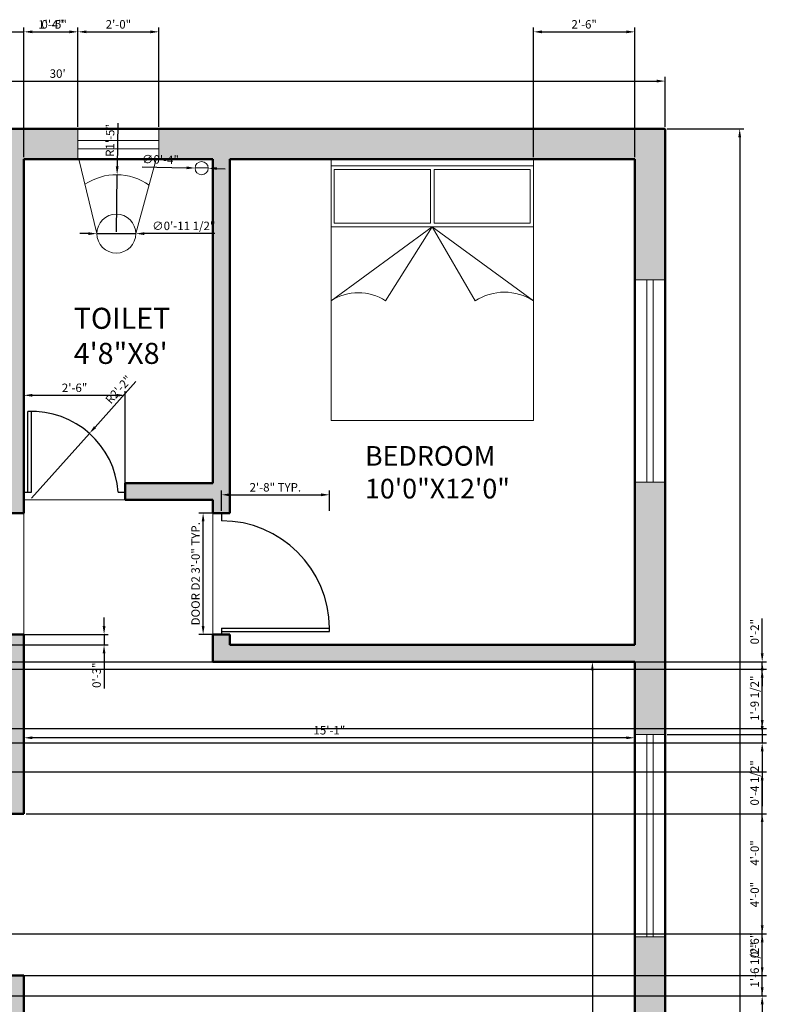
# Model space of a CAD drawing. Units: inches. Extents: x 457 to 882, y 0 to 1111.
# Tile 4 of 4: x 660 to 882, y 817 to 1109. Entities that reach past the tile are written whole.
import ezdxf

# ---------------------------------------------------------------- set-up
doc = ezdxf.new("R2010")
doc.units = ezdxf.units.IN
for name, color, linetype, lineweight in [('A-ANNO-DIMS', 2, 'Continuous', 18), ('A-AREA-IDEN', 7, 'Continuous', 25), ('A-DOOR', 3, 'Continuous', 25), ('A-DOOR-THRE', 8, 'Continuous', 13), ('A-FLOR-FIXT', 8, 'Continuous', 18), ('A-FURN', 8, 'Continuous', 18), ('A-GLAZ', 5, 'Continuous', 18), ('A-WALL', 7, 'Continuous', 50), ('A-WALL-PATT', 252, 'Continuous', 13)]:
    doc.layers.add(name, color=color, linetype=linetype, lineweight=lineweight)
doc.styles.get("Standard").update_dxf_attribs({"font": 'arial.ttf'})
doc.dimstyles.new('ISO-25', dxfattribs={"dimtxt": 2.5, "dimasz": 2.5, "dimexe": 1.25, "dimexo": 0.625, "dimtad": 1, "dimdec": 0, "dimlunit": 3, "dimtxsty": 'Standard', "dimcen": 2.5, "dimadec": 0, "dimazin": 0, "dimtfac": 1, "dimtdec": 0, "dimtmove": 0, "dimatfit": 3, "dimfxl": 1, "dimarcsym": 0})

# ---------------------------------------------------------------- blocks, each defined once
blk = doc.blocks.new('*D2')
at = {"layer": 'A-ANNO-DIMS', "color": 0, "lineweight": -2, "transparency": 16777216}
for p, q in [((491.26, 1077.13), (491.26, 1091.91)), ((851.26, 1077.13), (851.26, 1091.91)), ((493.76, 1090.66), (848.76, 1090.66))]:
    blk.add_line(p, q, dxfattribs=at)
at = {"layer": 'A-ANNO-DIMS', "color": 0, "transparency": 16777216}
for points in [[(493.76, 1091.08), (493.76, 1090.24), (491.26, 1090.66)], [(848.76, 1091.08), (848.76, 1090.24), (851.26, 1090.66)]]:
    blk.add_solid(points, dxfattribs=at)
at = {"layer": 'Defpoints', "color": 0, "transparency": 16777216}
for p in [(851.26, 1090.66), (491.26, 1076.51), (851.26, 1076.51)]:
    blk.add_point(p, dxfattribs=at)
at = {"layer": 'A-ANNO-DIMS', "color": 0, "transparency": 16777216, "insert": (671.26, 1092.56), "char_height": 2.5, "attachment_point": 5}
blk.add_mtext("30'", dxfattribs=at)
blk = doc.blocks.new('*D3')
at = {"layer": 'A-ANNO-DIMS', "color": 0, "lineweight": -2, "transparency": 16777216}
for p, q in [((851.88, 1076.51), (874.6, 1076.51)), ((873.35, 1074.01), (873.35, 539.01)), ((851.88, 536.51), (874.6, 536.51))]:
    blk.add_line(p, q, dxfattribs=at)
at = {"layer": 'A-ANNO-DIMS', "color": 0, "transparency": 16777216}
for points in [[(872.93, 1074.01), (873.76, 1074.01), (873.35, 1076.51)], [(872.93, 539.01), (873.76, 539.01), (873.35, 536.51)]]:
    blk.add_solid(points, dxfattribs=at)
at = {"layer": 'Defpoints', "color": 0, "transparency": 16777216}
for p in [(851.26, 1076.51), (851.26, 536.51), (873.35, 536.51)]:
    blk.add_point(p, dxfattribs=at)
at = {"layer": 'A-ANNO-DIMS', "color": 0, "transparency": 16777216, "insert": (871.45, 806.51), "char_height": 2.5, "attachment_point": 5, "rotation": 90}
blk.add_mtext("45'", dxfattribs=at)
blk = doc.blocks.new('*D6')
at = {"layer": 'A-ANNO-DIMS', "color": 0, "lineweight": -2, "transparency": 16777216}
for p, q in [((661.26, 917.88), (661.26, 894.76)), ((842.26, 917.88), (842.26, 894.76)), ((839.76, 896.01), (663.76, 896.01))]:
    blk.add_line(p, q, dxfattribs=at)
at = {"layer": 'A-ANNO-DIMS', "color": 0, "transparency": 16777216}
for points in [[(663.76, 896.42), (663.76, 895.59), (661.26, 896.01)], [(839.76, 896.42), (839.76, 895.59), (842.26, 896.01)]]:
    blk.add_solid(points, dxfattribs=at)
at = {"layer": 'Defpoints', "color": 0, "transparency": 16777216}
for p in [(661.26, 918.51), (842.26, 918.51), (661.26, 896.01)]:
    blk.add_point(p, dxfattribs=at)
at = {"layer": 'A-ANNO-DIMS', "color": 0, "transparency": 16777216, "insert": (751.76, 897.91), "char_height": 2.5, "attachment_point": 5}
blk.add_mtext('15\'-1"', dxfattribs=at)
blk = doc.blocks.new('*D7')
at = {"layer": 'A-ANNO-DIMS', "color": 0, "lineweight": -2, "transparency": 16777216}
for p, q in [((841.63, 918.51), (828.45, 918.51)), ((829.7, 916.01), (829.7, 631.01)), ((841.63, 628.51), (828.45, 628.51))]:
    blk.add_line(p, q, dxfattribs=at)
at = {"layer": 'A-ANNO-DIMS', "color": 0, "transparency": 16777216}
for points in [[(829.28, 916.01), (830.11, 916.01), (829.7, 918.51)], [(829.28, 631.01), (830.11, 631.01), (829.7, 628.51)]]:
    blk.add_solid(points, dxfattribs=at)
at = {"layer": 'Defpoints', "color": 0, "transparency": 16777216}
for p in [(842.26, 918.51), (829.7, 628.51), (842.26, 628.51)]:
    blk.add_point(p, dxfattribs=at)
at = {"layer": 'A-ANNO-DIMS', "color": 0, "transparency": 16777216, "insert": (827.82, 773.51), "char_height": 2.5, "attachment_point": 5, "rotation": 90}
blk.add_mtext('24\'-2"', dxfattribs=at)
blk = doc.blocks.new('BED-DOUBLE-60')
for p, q in [((0, 77.49), (0, 0)), ((60, 77.49), (0, 77.49)), ((60, 0), (60, 77.49)), ((60, 75.49), (0, 75.49)), ((29.44, 74.49), (0.94, 74.49)), ((0.94, 74.49), (0.94, 58.49)), ((29.44, 74.49), (29.44, 58.49)), ((59, 74.49), (30.53, 74.49)), ((30.53, 74.49), (30.53, 58.49)), ((59, 74.49), (59, 58.49)), ((29.44, 58.49), (0.94, 58.49)), ((59, 58.49), (30.53, 58.49)), ((60, 57.49), (0, 57.49)), ((30, 57.49), (0, 35.49)), ((30, 57.49), (16.16, 35.49)), ((60, 35.49), (30, 57.49)), ((30, 57.49), (42.73, 35.49)), ((0, 0), (60, 0))]:
    blk.add_line(p, q)
for centre, radius, start, end in [((51.36, 22.4), 15.69, 56.5972, 123.4028), ((8.08, 23.34), 14.59, 56.3669, 123.6331)]:
    blk.add_arc(centre, radius, start, end)
blk = doc.blocks.new('WIN-60-GLAZING')
for p, q in [((0, 0), (0, 60)), ((1.86, 0), (1.86, 60))]:
    blk.add_line(p, q)
blk = doc.blocks.new('DOOR-32-SWING')
for p, q in [((0, 36), (0, 33.7)), ((0, 1.85), (32, 1.85)), ((0, 1.85), (0, 0))]:
    blk.add_line(p, q)
blk.add_arc((0, 1.7), 32, 0.2643, 90)
blk = doc.blocks.new('*D20')
at = {"layer": 'A-ANNO-DIMS', "color": 0, "lineweight": -2, "transparency": 16777216}
for p, q in [((719.13, 962.63), (713.11, 962.63)), ((714.36, 929.13), (714.36, 960.13)), ((719.13, 926.63), (713.11, 926.63))]:
    blk.add_line(p, q, dxfattribs=at)
at = {"layer": 'A-ANNO-DIMS', "color": 0, "transparency": 16777216}
for points in [[(713.94, 960.13), (714.77, 960.13), (714.36, 962.63)], [(713.94, 929.13), (714.77, 929.13), (714.36, 926.63)]]:
    blk.add_solid(points, dxfattribs=at)
at = {"layer": 'Defpoints', "color": 0, "transparency": 16777216}
for p in [(714.36, 962.63), (719.76, 962.63), (719.76, 926.63)]:
    blk.add_point(p, dxfattribs=at)
at = {"layer": 'A-ANNO-DIMS', "color": 0, "transparency": 16777216, "insert": (712.44, 944.63), "char_height": 2.5, "attachment_point": 5, "rotation": 90}
blk.add_mtext('DOOR D2 3\'-0" TYP.', dxfattribs=at)
blk = doc.blocks.new('*D21')
at = {"layer": 'A-ANNO-DIMS', "color": 0, "lineweight": -2, "transparency": 16777216}
for p, q in [((719.76, 963.25), (719.76, 969.28)), ((751.76, 963.25), (751.76, 969.28)), ((722.26, 968.03), (749.26, 968.03))]:
    blk.add_line(p, q, dxfattribs=at)
at = {"layer": 'A-ANNO-DIMS', "color": 0, "transparency": 16777216}
for points in [[(722.26, 968.45), (722.26, 967.61), (719.76, 968.03)], [(749.26, 968.45), (749.26, 967.61), (751.76, 968.03)]]:
    blk.add_solid(points, dxfattribs=at)
at = {"layer": 'Defpoints', "color": 0, "transparency": 16777216}
for p in [(751.76, 968.03), (719.76, 962.63), (751.76, 962.63)]:
    blk.add_point(p, dxfattribs=at)
at = {"layer": 'A-ANNO-DIMS', "color": 0, "transparency": 16777216, "insert": (735.76, 969.93), "char_height": 2.5, "attachment_point": 5}
blk.add_mtext('2\'-8" TYP.', dxfattribs=at)
blk = doc.blocks.new('*D24')
at = {"layer": 'A-ANNO-DIMS', "color": 0, "lineweight": -2, "transparency": 16777216}
for p, q in [((661.26, 969.4), (661.26, 998.77)), ((691.26, 969.4), (691.26, 998.77)), ((663.76, 997.52), (688.76, 997.52))]:
    blk.add_line(p, q, dxfattribs=at)
at = {"layer": 'A-ANNO-DIMS', "color": 0, "transparency": 16777216}
for points in [[(663.76, 997.94), (663.76, 997.1), (661.26, 997.52)], [(688.76, 997.94), (688.76, 997.1), (691.26, 997.52)]]:
    blk.add_solid(points, dxfattribs=at)
at = {"layer": 'Defpoints', "color": 0, "transparency": 16777216}
for p in [(691.26, 997.52), (661.26, 968.77), (691.26, 968.77)]:
    blk.add_point(p, dxfattribs=at)
at = {"layer": 'A-ANNO-DIMS', "color": 0, "transparency": 16777216, "insert": (676.26, 999.42), "char_height": 2.5, "attachment_point": 5}
blk.add_mtext('2\'-6"', dxfattribs=at)
blk = doc.blocks.new('*D27')
at = {"layer": 'A-ANNO-DIMS', "color": 0, "lineweight": -2, "transparency": 16777216}
for p, q in [((685.01, 929.13), (685.01, 931.63)), ((656.88, 926.63), (686.26, 926.63)), ((685.01, 926.63), (685.01, 923.51)), ((656.88, 923.51), (686.26, 923.51)), ((685.01, 921.01), (685.01, 910.61))]:
    blk.add_line(p, q, dxfattribs=at)
at = {"layer": 'A-ANNO-DIMS', "color": 0, "transparency": 16777216}
for points in [[(684.59, 929.13), (685.42, 929.13), (685.01, 926.63)], [(684.59, 921.01), (685.42, 921.01), (685.01, 923.51)]]:
    blk.add_solid(points, dxfattribs=at)
at = {"layer": 'Defpoints', "color": 0, "transparency": 16777216}
for p in [(656.26, 926.63), (656.26, 923.51), (685.01, 923.51)]:
    blk.add_point(p, dxfattribs=at)
at = {"layer": 'A-ANNO-DIMS', "color": 0, "transparency": 16777216, "insert": (683.11, 914.56), "char_height": 2.5, "attachment_point": 5, "rotation": 90}
blk.add_mtext('0\'-3"', dxfattribs=at)
blk = doc.blocks.new('*D29')
at = {"layer": 'A-ANNO-DIMS', "color": 0, "lineweight": -2, "transparency": 16777216}
for p, q in [((656.26, 1068.13), (656.26, 1106.51)), ((661.26, 1068.13), (661.26, 1106.51)), ((653.76, 1105.26), (651.26, 1105.26)), ((656.26, 1105.26), (661.26, 1105.26)), ((663.76, 1105.26), (674.15, 1105.26))]:
    blk.add_line(p, q, dxfattribs=at)
at = {"layer": 'A-ANNO-DIMS', "color": 0, "transparency": 16777216}
for points in [[(653.76, 1105.67), (653.76, 1104.84), (656.26, 1105.26)], [(663.76, 1105.67), (663.76, 1104.84), (661.26, 1105.26)]]:
    blk.add_solid(points, dxfattribs=at)
at = {"layer": 'Defpoints', "color": 0, "transparency": 16777216}
for p in [(661.26, 1105.26), (656.26, 1067.51), (661.26, 1067.51)]:
    blk.add_point(p, dxfattribs=at)
at = {"layer": 'A-ANNO-DIMS', "color": 0, "transparency": 16777216, "insert": (670.21, 1107.16), "char_height": 2.5, "attachment_point": 5}
blk.add_mtext('0\'-5"', dxfattribs=at)
blk = doc.blocks.new('*D34')
at = {"layer": 'A-ANNO-DIMS', "color": 0, "lineweight": -2, "transparency": 16777216}
for p, q in [((842.88, 918.51), (881.26, 918.51)), ((880.01, 899.48), (880.01, 916.01)), ((851.88, 896.98), (881.26, 896.98))]:
    blk.add_line(p, q, dxfattribs=at)
at = {"layer": 'A-ANNO-DIMS', "color": 0, "transparency": 16777216}
for points in [[(879.59, 916.01), (880.42, 916.01), (880.01, 918.51)], [(879.59, 899.48), (880.42, 899.48), (880.01, 896.98)]]:
    blk.add_solid(points, dxfattribs=at)
at = {"layer": 'Defpoints', "color": 0, "transparency": 16777216}
for p in [(842.26, 918.51), (880.01, 918.51), (851.26, 896.98)]:
    blk.add_point(p, dxfattribs=at)
at = {"layer": 'A-ANNO-DIMS', "color": 0, "transparency": 16777216, "insert": (878.09, 907.74), "char_height": 2.5, "attachment_point": 5, "rotation": 90}
blk.add_mtext('1\'-9 1/2"', dxfattribs=at)
blk = doc.blocks.new('*D36')
at = {"layer": 'A-ANNO-DIMS', "color": 0, "lineweight": -2, "transparency": 16777216}
for p, q in [((661.26, 1068.13), (661.26, 1106.51)), ((677.26, 1077.13), (677.26, 1106.51)), ((663.76, 1105.26), (674.76, 1105.26))]:
    blk.add_line(p, q, dxfattribs=at)
at = {"layer": 'A-ANNO-DIMS', "color": 0, "transparency": 16777216}
for points in [[(663.76, 1105.67), (663.76, 1104.84), (661.26, 1105.26)], [(674.76, 1105.67), (674.76, 1104.84), (677.26, 1105.26)]]:
    blk.add_solid(points, dxfattribs=at)
at = {"layer": 'Defpoints', "color": 0, "transparency": 16777216}
for p in [(677.26, 1105.26), (677.26, 1076.51), (661.26, 1067.51)]:
    blk.add_point(p, dxfattribs=at)
at = {"layer": 'A-ANNO-DIMS', "color": 0, "transparency": 16777216, "insert": (669.26, 1107.14), "char_height": 2.5, "attachment_point": 5}
blk.add_mtext('1\'-4"', dxfattribs=at)
blk = doc.blocks.new('*D37')
at = {"layer": 'A-ANNO-DIMS', "color": 0, "lineweight": -2, "transparency": 16777216}
for p, q in [((677.26, 1077.13), (677.26, 1106.51)), ((701.26, 1077.13), (701.26, 1106.51)), ((679.76, 1105.26), (698.76, 1105.26))]:
    blk.add_line(p, q, dxfattribs=at)
at = {"layer": 'A-ANNO-DIMS', "color": 0, "transparency": 16777216}
for points in [[(679.76, 1105.67), (679.76, 1104.84), (677.26, 1105.26)], [(698.76, 1105.67), (698.76, 1104.84), (701.26, 1105.26)]]:
    blk.add_solid(points, dxfattribs=at)
at = {"layer": 'Defpoints', "color": 0, "transparency": 16777216}
for p in [(701.26, 1105.26), (677.26, 1076.51), (701.26, 1076.51)]:
    blk.add_point(p, dxfattribs=at)
at = {"layer": 'A-ANNO-DIMS', "color": 0, "transparency": 16777216, "insert": (689.26, 1107.16), "char_height": 2.5, "attachment_point": 5}
blk.add_mtext('2\'-0"', dxfattribs=at)
blk = doc.blocks.new('*D47')
at = {"layer": 'A-ANNO-DIMS', "color": 0, "lineweight": -2, "transparency": 16777216}
for p, q in [((661.88, 873.51), (881.26, 873.51)), ((880.01, 828.01), (880.01, 871.01)), ((661.88, 825.51), (881.26, 825.51))]:
    blk.add_line(p, q, dxfattribs=at)
at = {"layer": 'A-ANNO-DIMS', "color": 0, "transparency": 16777216}
for points in [[(879.59, 871.01), (880.42, 871.01), (880.01, 873.51)], [(879.59, 828.01), (880.42, 828.01), (880.01, 825.51)]]:
    blk.add_solid(points, dxfattribs=at)
at = {"layer": 'Defpoints', "color": 0, "transparency": 16777216}
for p in [(661.26, 873.51), (880.01, 873.51), (661.26, 825.51)]:
    blk.add_point(p, dxfattribs=at)
at = {"layer": 'A-ANNO-DIMS', "color": 0, "transparency": 16777216, "insert": (878.11, 849.51), "char_height": 2.5, "attachment_point": 5, "rotation": 90}
blk.add_mtext('4\'-0"', dxfattribs=at)
blk = doc.blocks.new('*D48')
at = {"layer": 'A-ANNO-DIMS', "color": 0, "lineweight": -2, "transparency": 16777216}
for p, q in [((880.01, 828.01), (880.01, 838.4)), ((656.88, 825.51), (881.26, 825.51)), ((880.01, 819.51), (880.01, 825.51)), ((656.88, 819.51), (881.26, 819.51)), ((880.01, 817.01), (880.01, 814.51))]:
    blk.add_line(p, q, dxfattribs=at)
at = {"layer": 'A-ANNO-DIMS', "color": 0, "transparency": 16777216}
for points in [[(879.59, 828.01), (880.42, 828.01), (880.01, 825.51)], [(879.59, 817.01), (880.42, 817.01), (880.01, 819.51)]]:
    blk.add_solid(points, dxfattribs=at)
at = {"layer": 'Defpoints', "color": 0, "transparency": 16777216}
for p in [(656.26, 825.51), (880.01, 825.51), (656.26, 819.51)]:
    blk.add_point(p, dxfattribs=at)
at = {"layer": 'A-ANNO-DIMS', "color": 0, "transparency": 16777216, "insert": (878.11, 834.45), "char_height": 2.5, "attachment_point": 5, "rotation": 90}
blk.add_mtext('0\'-6"', dxfattribs=at)
blk = doc.blocks.new('*D50')
at = {"layer": 'A-ANNO-DIMS', "color": 0, "lineweight": -2, "transparency": 16777216}
for p, q in [((527.99, 885.87), (881.26, 885.87)), ((880.01, 840.37), (880.01, 883.37)), ((527.99, 837.87), (881.26, 837.87))]:
    blk.add_line(p, q, dxfattribs=at)
at = {"layer": 'A-ANNO-DIMS', "color": 0, "transparency": 16777216}
for points in [[(879.59, 883.37), (880.42, 883.37), (880.01, 885.87)], [(879.59, 840.37), (880.42, 840.37), (880.01, 837.87)]]:
    blk.add_solid(points, dxfattribs=at)
at = {"layer": 'Defpoints', "color": 0, "transparency": 16777216}
for p in [(527.36, 885.87), (880.01, 885.87), (527.36, 837.87)]:
    blk.add_point(p, dxfattribs=at)
at = {"layer": 'A-ANNO-DIMS', "color": 0, "transparency": 16777216, "insert": (878.11, 861.87), "char_height": 2.5, "attachment_point": 5, "rotation": 90}
blk.add_mtext('4\'-0"', dxfattribs=at)
blk = doc.blocks.new('*D51')
at = {"layer": 'A-ANNO-DIMS', "color": 0, "lineweight": -2, "transparency": 16777216}
for p, q in [((503.99, 837.87), (881.26, 837.87)), ((880.01, 822.01), (880.01, 835.37)), ((500.88, 819.51), (881.26, 819.51))]:
    blk.add_line(p, q, dxfattribs=at)
at = {"layer": 'A-ANNO-DIMS', "color": 0, "transparency": 16777216}
for points in [[(879.59, 835.37), (880.42, 835.37), (880.01, 837.87)], [(879.59, 822.01), (880.42, 822.01), (880.01, 819.51)]]:
    blk.add_solid(points, dxfattribs=at)
at = {"layer": 'Defpoints', "color": 0, "transparency": 16777216}
for p in [(503.36, 837.87), (880.01, 837.87), (500.26, 819.51)]:
    blk.add_point(p, dxfattribs=at)
at = {"layer": 'A-ANNO-DIMS', "color": 0, "transparency": 16777216, "insert": (878.09, 828.69), "char_height": 2.5, "attachment_point": 5, "rotation": 90}
blk.add_mtext('1\'-6 1/2"', dxfattribs=at)
blk = doc.blocks.new('*D55')
at = {"layer": 'A-ANNO-DIMS', "color": 0, "lineweight": -2, "transparency": 16777216}
for p, q in [((880.01, 921.01), (880.01, 931.4)), ((656.88, 918.51), (881.26, 918.51)), ((880.01, 916.3), (880.01, 918.51)), ((598.94, 916.3), (881.26, 916.3)), ((880.01, 913.8), (880.01, 911.3))]:
    blk.add_line(p, q, dxfattribs=at)
at = {"layer": 'A-ANNO-DIMS', "color": 0, "transparency": 16777216}
for points in [[(879.59, 921.01), (880.42, 921.01), (880.01, 918.51)], [(879.59, 913.8), (880.42, 913.8), (880.01, 916.3)]]:
    blk.add_solid(points, dxfattribs=at)
at = {"layer": 'Defpoints', "color": 0, "transparency": 16777216}
for p in [(656.26, 918.51), (880.01, 918.51), (598.31, 916.3)]:
    blk.add_point(p, dxfattribs=at)
at = {"layer": 'A-ANNO-DIMS', "color": 0, "transparency": 16777216, "insert": (878.11, 927.45), "char_height": 2.5, "attachment_point": 5, "rotation": 90}
blk.add_mtext('0\'-2"', dxfattribs=at)
blk = doc.blocks.new('*D57')
at = {"layer": 'A-ANNO-DIMS', "color": 0, "lineweight": -2, "transparency": 16777216}
for p, q in [((880.01, 901.27), (880.01, 903.77)), ((610.53, 898.77), (881.26, 898.77)), ((880.01, 898.77), (880.01, 894.51)), ((656.88, 894.51), (881.26, 894.51)), ((880.01, 892.01), (880.01, 875.78))]:
    blk.add_line(p, q, dxfattribs=at)
at = {"layer": 'A-ANNO-DIMS', "color": 0, "transparency": 16777216}
for points in [[(879.59, 901.27), (880.42, 901.27), (880.01, 898.77)], [(879.59, 892.01), (880.42, 892.01), (880.01, 894.51)]]:
    blk.add_solid(points, dxfattribs=at)
at = {"layer": 'Defpoints', "color": 0, "transparency": 16777216}
for p in [(609.9, 898.77), (656.26, 894.51), (880.01, 894.51)]:
    blk.add_point(p, dxfattribs=at)
at = {"layer": 'A-ANNO-DIMS', "color": 0, "transparency": 16777216, "insert": (878.09, 882.64), "char_height": 2.5, "attachment_point": 5, "rotation": 90}
blk.add_mtext('0\'-4 1/2"', dxfattribs=at)
blk = doc.blocks.new('*D59')
at = {"layer": 'A-ANNO-DIMS', "color": 0, "lineweight": -2, "transparency": 16777216}
for p, q in [((812.26, 1068.13), (812.26, 1106.51)), ((842.26, 1068.13), (842.26, 1106.51)), ((814.76, 1105.26), (839.76, 1105.26))]:
    blk.add_line(p, q, dxfattribs=at)
at = {"layer": 'A-ANNO-DIMS', "color": 0, "transparency": 16777216}
for points in [[(814.76, 1105.67), (814.76, 1104.84), (812.26, 1105.26)], [(839.76, 1105.67), (839.76, 1104.84), (842.26, 1105.26)]]:
    blk.add_solid(points, dxfattribs=at)
at = {"layer": 'Defpoints', "color": 0, "transparency": 16777216}
for p in [(842.26, 1105.26), (812.26, 1067.51), (842.26, 1067.51)]:
    blk.add_point(p, dxfattribs=at)
at = {"layer": 'A-ANNO-DIMS', "color": 0, "transparency": 16777216, "insert": (827.26, 1107.16), "char_height": 2.5, "attachment_point": 5}
blk.add_mtext('2\'-6"', dxfattribs=at)
blk = doc.blocks.new('*D62')
at = {"layer": 'A-ANNO-DIMS', "color": 0, "lineweight": -2, "transparency": 16777216}
for p, q in [((694.39, 1001.58), (682.33, 988.08)), ((663.49, 967), (680.66, 986.22))]:
    blk.add_line(p, q, dxfattribs=at)
at = {"layer": 'A-ANNO-DIMS', "color": 0, "transparency": 16777216}
blk.add_solid([(682.02, 988.36), (682.64, 987.8), (680.66, 986.22)], dxfattribs=at)
at = {"layer": 'Defpoints', "color": 0, "transparency": 16777216}
for p in [(680.66, 986.22), (663.49, 967)]:
    blk.add_point(p, dxfattribs=at)
at = {"layer": 'A-ANNO-DIMS', "color": 0, "transparency": 16777216, "insert": (689.56, 999), "char_height": 2.5, "attachment_point": 5, "rotation": 48.2111}
blk.add_mtext('R2\'-2"', dxfattribs=at)
blk = doc.blocks.new('*D65')
at = {"layer": 'A-ANNO-DIMS', "color": 0, "lineweight": -2, "transparency": 16777216}
for p, q in [((680.36, 1045.45), (677.86, 1045.45)), ((682.86, 1045.45), (694.42, 1045.45)), ((717.81, 1045.45), (696.92, 1045.45))]:
    blk.add_line(p, q, dxfattribs=at)
at = {"layer": 'A-ANNO-DIMS', "color": 0, "transparency": 16777216}
for points in [[(680.36, 1045.86), (680.36, 1045.03), (682.86, 1045.45)], [(696.92, 1045.86), (696.92, 1045.03), (694.42, 1045.45)]]:
    blk.add_solid(points, dxfattribs=at)
at = {"layer": 'Defpoints', "color": 0, "transparency": 16777216}
for p in [(682.86, 1045.45), (694.42, 1045.45)]:
    blk.add_point(p, dxfattribs=at)
at = {"layer": 'A-ANNO-DIMS', "color": 0, "transparency": 16777216, "insert": (708.62, 1047.42), "char_height": 2.5, "attachment_point": 5, "rotation": 0.0005}
blk.add_mtext('∅0\'-11 1/2"', dxfattribs=at)
blk = doc.blocks.new('*D66')
at = {"layer": 'A-ANNO-DIMS', "color": 0, "lineweight": -2, "transparency": 16777216}
for p, q in [((689.06, 1078.18), (688.9, 1065.39)), ((688.65, 1046.02), (688.87, 1062.9))]:
    blk.add_line(p, q, dxfattribs=at)
at = {"layer": 'A-ANNO-DIMS', "color": 0, "transparency": 16777216}
blk.add_solid([(688.48, 1065.4), (689.32, 1065.39), (688.87, 1062.9)], dxfattribs=at)
at = {"layer": 'Defpoints', "color": 0, "transparency": 16777216}
for p in [(688.87, 1062.9), (688.65, 1046.02)]:
    blk.add_point(p, dxfattribs=at)
at = {"layer": 'A-ANNO-DIMS', "color": 0, "transparency": 16777216, "insert": (687.1, 1073.06), "char_height": 2.5, "attachment_point": 5, "rotation": 89.2668}
blk.add_mtext('R1\'-5"', dxfattribs=at)
blk = doc.blocks.new('*D67')
at = {"layer": 'A-ANNO-DIMS', "color": 0, "lineweight": -2, "transparency": 16777216}
for p, q in [((696.34, 1065.25), (709.46, 1064.96)), ((715.88, 1064.81), (711.96, 1064.9)), ((718.38, 1064.76), (720.88, 1064.7))]:
    blk.add_line(p, q, dxfattribs=at)
at = {"layer": 'A-ANNO-DIMS', "color": 0, "transparency": 16777216}
for points in [[(709.47, 1065.37), (709.45, 1064.54), (711.96, 1064.9)], [(718.39, 1065.18), (718.37, 1064.34), (715.88, 1064.81)]]:
    blk.add_solid(points, dxfattribs=at)
at = {"layer": 'Defpoints', "color": 0, "transparency": 16777216}
for p in [(711.96, 1064.9), (715.88, 1064.81)]:
    blk.add_point(p, dxfattribs=at)
at = {"layer": 'A-ANNO-DIMS', "color": 0, "transparency": 16777216, "insert": (701.69, 1067.1), "char_height": 2.5, "attachment_point": 5, "rotation": 358.7346}
blk.add_mtext('∅0\'-4"', dxfattribs=at)

msp = doc.modelspace()

# ---------------------------------------------------------------- hatches: boundary and pattern name
at = {"layer": 'A-WALL-PATT'}
h = msp.add_hatch(color=256, dxfattribs=at)
h.dxf.hatch_style = 1
h.paths.add_polyline_path([(677.26, 1076.51), (491.26, 1076.51), (491.26, 1031.73), (500.26, 1031.73), (500.26, 1067.51), (656.26, 1067.51), (656.26, 962.63), (661.26, 962.63), (661.26, 1067.51), (677.26, 1067.51)])
h.paths.add_polyline_path([(851.26, 1076.51), (701.26, 1076.51), (701.26, 1067.51), (717.26, 1067.51), (717.26, 971.51), (691.26, 971.51), (691.26, 966.51), (717.26, 966.51), (717.26, 962.63), (722.26, 962.63), (722.26, 1067.51), (842.26, 1067.51), (842.26, 1031.73), (851.26, 1031.73)])
h.paths.add_polyline_path([(851.26, 971.73), (842.26, 971.73), (842.26, 923.51), (722.26, 923.51), (722.26, 926.63), (717.26, 926.63), (717.26, 918.51), (842.26, 918.51), (842.26, 896.98), (851.26, 896.98)])
h.paths.add_polyline_path([(661.26, 926.63), (656.26, 926.63), (656.26, 923.51), (500.26, 923.51), (500.26, 971.73), (491.26, 971.73), (491.26, 899.01), (500.26, 899.01), (500.26, 918.51), (656.26, 918.51), (656.26, 873.51), (661.26, 873.51)])
h.paths.add_polyline_path([(500.26, 839.01), (491.26, 839.01), (491.26, 778.51), (500.26, 778.51), (500.26, 814.51), (656.26, 814.51), (656.26, 726.51), (661.26, 726.51), (661.26, 825.51), (656.26, 825.51), (656.26, 819.51), (500.26, 819.51)])
h.paths.add_polyline_path([(661.26, 633.51), (656.26, 633.51), (656.26, 545.51), (606.26, 545.51), (606.26, 536.51), (661.26, 536.51)], flags=0)
h.paths.add_polyline_path([(851.26, 560.51), (842.26, 560.51), (842.26, 545.51), (721.26, 545.51), (721.26, 536.51), (851.26, 536.51)])
h.paths.add_polyline_path([(851.26, 649.3), (842.26, 649.3), (842.26, 628.51), (700.26, 628.51), (700.26, 623.51), (842.26, 623.51), (842.26, 608.51), (851.26, 608.51)])
h.paths.add_polyline_path([(500.26, 677.51), (656.26, 677.51), (656.26, 671.51), (661.26, 671.51), (661.26, 688.51), (656.26, 688.51), (656.26, 682.51), (500.26, 682.51), (500.26, 718.51), (491.26, 718.51), (491.26, 536.51), (546.26, 536.51), (546.26, 545.51), (500.26, 545.51)])
h = msp.add_hatch(color=256, dxfattribs=at)
h.dxf.hatch_style = 1
h.paths.add_polyline_path([(851.26, 836.98), (842.26, 836.98), (842.26, 709.3), (851.26, 709.3)])

# ---------------------------------------------------------------- linework, layer by layer
at = {"layer": 'A-DOOR'}
for p, q in [((662.37, 968.77), (662.37, 992.77)), ((663.49, 968.77), (663.49, 992.77)), ((661.26, 968.77), (663.49, 968.77)), ((689.2, 968.77), (691.26, 968.77)), ((751.76, 927.55), (751.76, 928.48)), ((719.76, 927.55), (751.76, 927.55))]:
    msp.add_line(p, q, dxfattribs=at)
msp.add_arc((663.49, 967), 25.77, 3.9421, 92.4792, dxfattribs=at)
at = {"layer": 'A-DOOR-THRE'}
for p, q in [((691.26, 966.51), (661.26, 966.51)), ((661.26, 962.63), (661.26, 926.63)), ((717.26, 962.63), (717.26, 926.63))]:
    msp.add_line(p, q, dxfattribs=at)
at = {"layer": 'A-FLOR-FIXT'}
for p, q in [((682.86, 1045.45), (677.48, 1067.51)), ((694.42, 1045.45), (700.47, 1067.51))]:
    msp.add_line(p, q, dxfattribs=at)
for centre, radius in [((713.92, 1064.86), 1.96), ((688.64, 1045.45), 5.78)]:
    msp.add_circle(centre, radius, dxfattribs=at)
msp.add_arc((688.65, 1046.02), 16.88, 54.866, 123.6705, dxfattribs=at)
at = {"layer": 'A-GLAZ'}
for p, q in [((677.26, 1076.51), (677.26, 1067.51)), ((701.26, 1067.51), (701.26, 1076.51)), ((701.26, 1073.08), (677.26, 1073.08)), ((701.26, 1070.61), (677.26, 1070.61)), ((851.26, 1031.73), (842.26, 1031.73)), ((842.26, 971.73), (851.26, 971.73)), ((851.26, 896.98), (842.26, 896.98)), ((842.26, 836.98), (851.26, 836.98))]:
    msp.add_line(p, q, dxfattribs=at)
at = {"layer": 'A-WALL'}
for p, q in [((851.26, 1076.51), (491.26, 1076.51)), ((851.26, 536.51), (851.26, 1076.51)), ((661.26, 1067.51), (661.26, 962.63)), ((717.26, 1067.51), (661.26, 1067.51)), ((717.26, 971.51), (717.26, 1067.51)), ((842.26, 1067.51), (722.26, 1067.51)), ((722.26, 962.63), (722.26, 1067.51)), ((842.26, 923.51), (842.26, 1067.51)), ((717.26, 971.51), (691.26, 971.51)), ((691.26, 966.51), (691.26, 971.51)), ((717.26, 966.51), (691.26, 966.51)), ((717.26, 966.51), (717.26, 962.63)), ((661.26, 962.63), (656.26, 962.63)), ((722.26, 962.63), (717.26, 962.63)), ((661.26, 926.63), (656.26, 926.63)), ((661.26, 926.63), (661.26, 873.51)), ((717.26, 918.51), (717.26, 926.63)), ((722.26, 926.63), (717.26, 926.63)), ((722.26, 923.51), (722.26, 926.63)), ((842.26, 923.51), (722.26, 923.51)), ((842.26, 918.51), (717.26, 918.51)), ((842.26, 628.51), (842.26, 918.51)), ((656.26, 873.51), (661.26, 873.51)), ((656.26, 825.51), (661.26, 825.51)), ((661.26, 825.51), (661.26, 726.51))]:
    msp.add_line(p, q, dxfattribs=at)

# ---------------------------------------------------------------- block references
at = {"layer": 'A-DOOR'}
msp.add_blockref('DOOR-32-SWING', (719.76, 926.63), dxfattribs=at)
at = {"layer": 'A-FURN'}
msp.add_blockref('BED-DOUBLE-60', (752.26, 990.01), dxfattribs=at)
at = {"layer": 'A-GLAZ'}
for p in [(845.86, 971.73), (845.86, 836.98)]:
    msp.add_blockref('WIN-60-GLAZING', p, dxfattribs=at)

# ---------------------------------------------------------------- texts
at = {"layer": 'A-AREA-IDEN', "attachment_point": 1}
for s, width, gutter_width, insert, char_height in [('TOILET\\P4\'8"X8\'', 110.1262, 31.2, (676.01, 1023.47), 6.24), ('BEDROOM\\P10\'0"X12\'0"', 35.0861, 29.11, (762.32, 982.48), 5.8229)]:
    msp.add_mtext_dynamic_manual_height_columns(s, width=width, gutter_width=gutter_width, heights=[0], dxfattribs=dict(at, insert=insert, char_height=char_height))

# ---------------------------------------------------------------- dimensions: what is measured, and where the dimension line sits
at = {"layer": 'A-ANNO-DIMS'}
for base, p1, p2, override, picture, middle in [((661.26, 1105.26), (656.26, 1067.51), (661.26, 1067.51), {"dimdec": 1, "dimlfac": 1, "dimrnd": 0, "dimzin": 1, "dimdsep": 46, "dimlunit": 4, "dimfrac": 2}, '*D29', (670.21, 1107.16)), ((677.26, 1105.26), (661.26, 1067.51), (677.26, 1076.51), {"dimdec": 1, "dimlfac": 1, "dimrnd": 0, "dimzin": 1, "dimdsep": 46, "dimlunit": 4, "dimfrac": 2}, '*D36', (669.26, 1107.14)), ((701.26, 1105.26), (677.26, 1076.51), (701.26, 1076.51), {"dimdec": 1, "dimlfac": 1, "dimrnd": 0, "dimzin": 1, "dimdsep": 46, "dimlunit": 4, "dimfrac": 2}, '*D37', (689.26, 1107.16)), ((842.26, 1105.26), (812.26, 1067.51), (842.26, 1067.51), {"dimdec": 1, "dimlfac": 1, "dimrnd": 0, "dimzin": 1, "dimdsep": 46, "dimlunit": 4, "dimfrac": 2}, '*D59', (827.26, 1107.16)), ((851.26, 1090.66), (491.26, 1076.51), (851.26, 1076.51), {"dimclrd": 0, "dimclre": 0, "dimclrt": 0}, '*D2', (671.26, 1092.56)), ((691.26, 997.52), (661.26, 968.77), (691.26, 968.77), {"dimdec": 1, "dimlfac": 1, "dimrnd": 0, "dimzin": 1, "dimdsep": 46, "dimlunit": 4, "dimfrac": 2}, '*D24', (676.26, 999.42)), ((661.26, 896.01), (842.26, 918.51), (661.26, 918.51), {"dimclrd": 0, "dimclre": 0, "dimclrt": 0}, '*D6', (751.76, 897.91))]:
    dim = msp.add_linear_dim(base=base, p1=p1, p2=p2, dimstyle='ISO-25', override=override, dxfattribs=at)
    dim.commit()
    dim.dimension.update_dxf_attribs({"geometry": picture, "text_midpoint": middle})
dim = msp.add_radius_dim(center=(688.65, 1046.02), mpoint=(688.87, 1062.9), dimstyle='ISO-25', override={"dimdec": 1, "dimlfac": 1, "dimrnd": 0, "dimzin": 1, "dimdsep": 46, "dimlunit": 4, "dimfrac": 2}, dxfattribs=at)
dim.commit()
dim.dimension.update_dxf_attribs({"geometry": '*D66', "text_midpoint": (687.1, 1073.06)})
for base, p1, p2, angle, override, picture, middle in [((873.35, 536.51), (851.26, 1076.51), (851.26, 536.51), 90, {"dimclrd": 0, "dimclre": 0, "dimclrt": 0}, '*D3', (871.45, 806.51)), ((880.01, 918.51), (598.31, 916.3), (656.26, 918.51), 90, {"dimdec": 1, "dimlfac": 1, "dimrnd": 0, "dimzin": 1, "dimdsep": 46, "dimlunit": 4, "dimfrac": 2}, '*D55', (878.11, 927.45)), ((685.01, 923.51), (656.26, 926.63), (656.26, 923.51), 270, {"dimdec": 1, "dimlfac": 1, "dimrnd": 0, "dimzin": 1, "dimdsep": 46, "dimlunit": 4, "dimfrac": 2}, '*D27', (683.11, 914.56)), ((829.7, 628.51), (842.26, 918.51), (842.26, 628.51), 90, {"dimclrd": 0, "dimclre": 0, "dimclrt": 0}, '*D7', (827.82, 773.51)), ((880.01, 918.51), (851.26, 896.98), (842.26, 918.51), 90, {"dimdec": 1, "dimlfac": 1, "dimrnd": 0, "dimzin": 1, "dimdsep": 46, "dimlunit": 4, "dimfrac": 2}, '*D34', (878.09, 907.74)), ((880.01, 894.51), (609.9, 898.77), (656.26, 894.51), 90, {"dimdec": 1, "dimlfac": 1, "dimrnd": 0, "dimzin": 1, "dimdsep": 46, "dimlunit": 4, "dimfrac": 2}, '*D57', (878.09, 882.64)), ((880.01, 885.87), (527.36, 837.87), (527.36, 885.87), 90, {"dimdec": 1, "dimlfac": 1, "dimrnd": 0, "dimzin": 1, "dimdsep": 46, "dimlunit": 4, "dimfrac": 2}, '*D50', (878.11, 861.87)), ((880.01, 873.51), (661.26, 825.51), (661.26, 873.51), 90, {"dimdec": 1, "dimlfac": 1, "dimrnd": 0, "dimzin": 1, "dimdsep": 46, "dimlunit": 4, "dimfrac": 2}, '*D47', (878.11, 849.51)), ((880.01, 837.87), (500.26, 819.51), (503.36, 837.87), 90, {"dimdec": 1, "dimlfac": 1, "dimrnd": 0, "dimzin": 1, "dimdsep": 46, "dimlunit": 4, "dimfrac": 2}, '*D51', (878.09, 828.69)), ((880.01, 825.51), (656.26, 819.51), (656.26, 825.51), 90, {"dimdec": 1, "dimlfac": 1, "dimrnd": 0, "dimzin": 1, "dimdsep": 46, "dimlunit": 4, "dimfrac": 2}, '*D48', (878.11, 834.45))]:
    dim = msp.add_linear_dim(base=base, p1=p1, p2=p2, angle=angle, dimstyle='ISO-25', override=override, dxfattribs=at)
    dim.commit()
    dim.dimension.update_dxf_attribs({"geometry": picture, "text_midpoint": middle})
dim = msp.add_diameter_dim_2p(p1=(715.88, 1064.81), p2=(711.96, 1064.9), dimstyle='ISO-25', override={"dimdec": 1, "dimlfac": 1, "dimrnd": 0, "dimzin": 1, "dimdsep": 46, "dimlunit": 4, "dimfrac": 2}, dxfattribs=at)
dim.commit()
dim.dimension.update_dxf_attribs({"geometry": '*D67', "text_midpoint": (701.65, 1065.13)})
dim = msp.add_diameter_dim_2p(p1=(682.86, 1045.45), p2=(694.42, 1045.45), dimstyle='ISO-25', override={"dimdec": 1, "dimlfac": 1, "dimrnd": 0, "dimzin": 1, "dimdsep": 46, "dimlunit": 4, "dimfrac": 2}, dxfattribs=at)
dim.commit()
dim.dimension.update_dxf_attribs({"geometry": '*D65', "text_midpoint": (708.62, 1045.45), "dimtype": 163})
dim = msp.add_radius_dim(center=(663.49, 967), mpoint=(680.66, 986.22), dimstyle='ISO-25', override={"dimdec": 1, "dimlfac": 1, "dimrnd": 0, "dimzin": 1, "dimdsep": 46, "dimlunit": 4, "dimfrac": 2}, dxfattribs=at)
dim.commit()
dim.dimension.update_dxf_attribs({"geometry": '*D62', "text_midpoint": (690.97, 997.74), "dimtype": 164})
dim = msp.add_linear_dim(base=(751.76, 968.03), p1=(719.76, 962.63), p2=(751.76, 962.63), text='<> TYP.', dimstyle='ISO-25', override={"dimdec": 1, "dimlfac": 1, "dimrnd": 0, "dimzin": 1, "dimdsep": 46, "dimlunit": 4, "dimfrac": 2}, dxfattribs=at)
dim.commit()
dim.dimension.update_dxf_attribs({"geometry": '*D21', "text_midpoint": (735.76, 969.93)})
dim = msp.add_linear_dim(base=(714.36, 962.63), p1=(719.76, 926.63), p2=(719.76, 962.63), angle=90, text='DOOR D2 <> TYP.', dimstyle='ISO-25', override={"dimdec": 1, "dimlfac": 1, "dimrnd": 0, "dimzin": 1, "dimdsep": 46, "dimlunit": 4, "dimfrac": 2}, dxfattribs=at)
dim.commit()
dim.dimension.update_dxf_attribs({"geometry": '*D20', "text_midpoint": (712.44, 944.63)})

doc.saveas('drawing.dxf')
